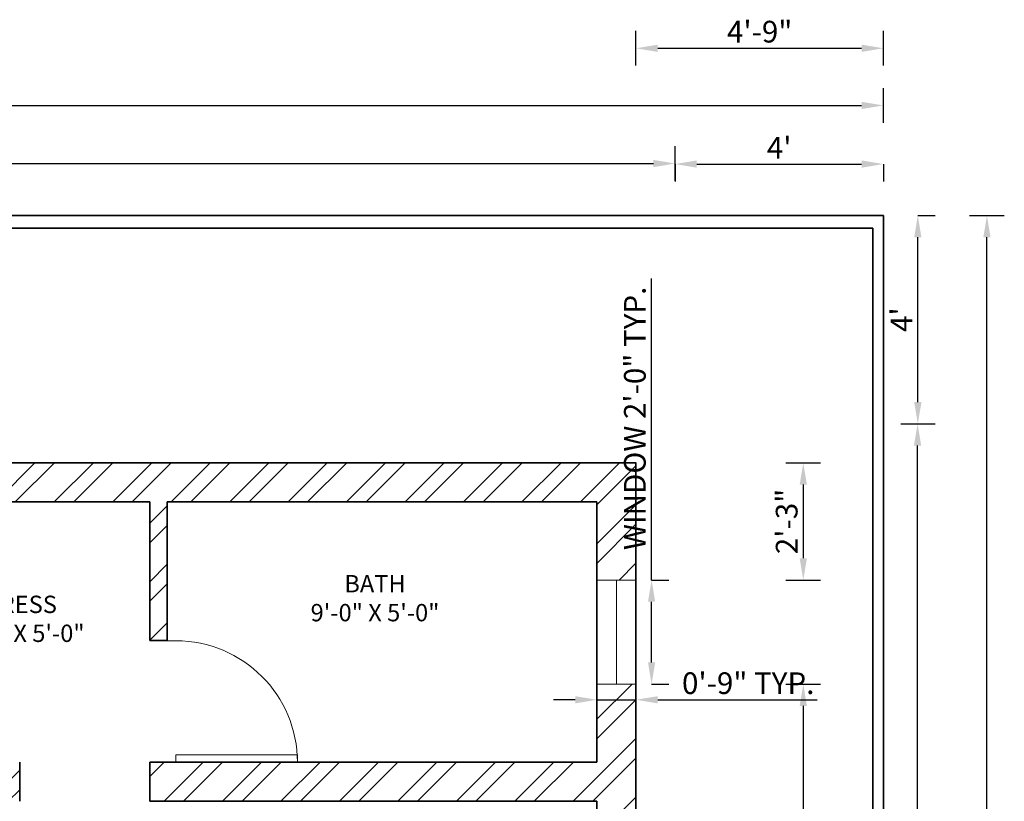
# Model space of a CAD drawing. Units: inches. Extents: x 468 to 1096, y 138 to 946.
# Tile 6 of 6: x 854 to 1081, y 766 to 946. Entities that reach past the tile are written whole.
import ezdxf

# ---------------------------------------------------------------- set-up
doc = ezdxf.new("R2010")
doc.units = ezdxf.units.IN
for name, color, linetype, lineweight in [('A-ANNO-DIMS', 2, 'Continuous', 18), ('A-AREA-IDEN', 7, 'Continuous', 18), ('A-DOOR', 3, 'Continuous', 18), ('A-GLAZ', 4, 'Continuous', 18), ('A-WALL', 7, 'Continuous', 35), ('A-WALL-PATT', 8, 'Continuous', 13), ('C-PROP', 7, 'Continuous', 35)]:
    doc.layers.add(name, color=color, linetype=linetype, lineweight=lineweight)
doc.styles.get("Standard").update_dxf_attribs({"font": 'arial.ttf'})
doc.dimstyles.new('ISO-25', dxfattribs={"dimtxt": 5, "dimasz": 5, "dimexe": 4, "dimexo": 4, "dimtad": 1, "dimdec": 1, "dimlunit": 3, "dimtxsty": 'Standard', "dimcen": 2.5, "dimadec": 0, "dimazin": 0, "dimtfac": 1, "dimtdec": 1, "dimtmove": 0, "dimatfit": 3, "dimfxl": 4, "dimfxlon": 1, "dimarcsym": 0})

# ---------------------------------------------------------------- blocks, each defined once
blk = doc.blocks.new('*U6')
for p, q in [((-28, 0), (-28, -6)), ((0, 0), (0, -6))]:
    blk.add_line(p, q)
blk.add_lwpolyline([(0, 0), (0, 28), (-1.75, 28), (-1.75, 0)], close=True)
blk.add_arc((0, 0), 28, 90, 180)
blk = doc.blocks.new('*D16')
at = {"layer": 'A-ANNO-DIMS', "color": 0, "lineweight": -2, "transparency": 16777216}
for p, q in [((639.13, 909.15), (639.13, 917.15)), ((1005.13, 909.15), (1005.13, 917.15)), ((644.13, 913.15), (1000.13, 913.15))]:
    blk.add_line(p, q, dxfattribs=at)
at = {"layer": 'A-ANNO-DIMS', "color": 0, "transparency": 16777216}
for points in [[(644.13, 913.98), (644.13, 912.31), (639.13, 913.15)], [(1000.13, 913.98), (1000.13, 912.31), (1005.13, 913.15)]]:
    blk.add_solid(points, dxfattribs=at)
at = {"layer": 'Defpoints', "color": 0, "transparency": 16777216}
for p in [(1005.13, 913.15), (639.13, 901.16), (1005.13, 901.16)]:
    blk.add_point(p, dxfattribs=at)
at = {"layer": 'A-ANNO-DIMS', "color": 0, "transparency": 16777216, "insert": (822.13, 916.33), "char_height": 5, "attachment_point": 5}
blk.add_mtext('30\'-6"', dxfattribs=at)
blk = doc.blocks.new('*D17')
at = {"layer": 'A-ANNO-DIMS', "color": 0, "lineweight": -2, "transparency": 16777216}
for p, q in [((1005.13, 913.03), (1005.13, 909.03)), ((1010.13, 913.03), (1048.13, 913.03)), ((1053.13, 913.03), (1053.13, 909.03))]:
    blk.add_line(p, q, dxfattribs=at)
at = {"layer": 'A-ANNO-DIMS', "color": 0, "transparency": 16777216}
for points in [[(1010.13, 913.86), (1010.13, 912.19), (1005.13, 913.03)], [(1048.13, 913.86), (1048.13, 912.19), (1053.13, 913.03)]]:
    blk.add_solid(points, dxfattribs=at)
at = {"layer": 'Defpoints', "color": 0, "transparency": 16777216}
for p in [(1005.13, 913.15), (1053.13, 913.15), (1053.13, 913.03)]:
    blk.add_point(p, dxfattribs=at)
at = {"layer": 'A-ANNO-DIMS', "color": 0, "transparency": 16777216, "insert": (1029.13, 916.15), "char_height": 5, "attachment_point": 5}
blk.add_mtext("4'", dxfattribs=at)
blk = doc.blocks.new('*D26')
at = {"layer": 'A-ANNO-DIMS', "color": 0, "lineweight": -2, "transparency": 16777216}
for p, q in [((1073, 901.16), (1081, 901.16)), ((1077, 186.16), (1077, 896.16)), ((1073, 181.16), (1081, 181.16))]:
    blk.add_line(p, q, dxfattribs=at)
at = {"layer": 'A-ANNO-DIMS', "color": 0, "transparency": 16777216}
for points in [[(1076.17, 896.16), (1077.83, 896.16), (1077, 901.16)], [(1076.17, 186.16), (1077.83, 186.16), (1077, 181.16)]]:
    blk.add_solid(points, dxfattribs=at)
at = {"layer": 'Defpoints', "color": 0, "transparency": 16777216}
for p in [(1053.13, 901.16), (1077, 901.16), (1053.13, 181.16)]:
    blk.add_point(p, dxfattribs=at)
at = {"layer": 'A-ANNO-DIMS', "color": 0, "transparency": 16777216, "insert": (1073.82, 541.16), "char_height": 5, "attachment_point": 5, "rotation": 90}
blk.add_mtext("60'", dxfattribs=at)
blk = doc.blocks.new('*D28')
at = {"layer": 'A-ANNO-DIMS', "color": 0, "lineweight": -2, "transparency": 16777216}
for p, q in [((1057.13, 853.16), (1065.02, 853.16)), ((1061.02, 417.16), (1061.02, 848.16)), ((1057.13, 412.16), (1065.02, 412.16))]:
    blk.add_line(p, q, dxfattribs=at)
at = {"layer": 'A-ANNO-DIMS', "color": 0, "transparency": 16777216}
for points in [[(1060.18, 848.16), (1061.85, 848.16), (1061.02, 853.16)], [(1060.18, 417.16), (1061.85, 417.16), (1061.02, 412.16)]]:
    blk.add_solid(points, dxfattribs=at)
at = {"layer": 'Defpoints', "color": 0, "transparency": 16777216}
for p in [(1053.13, 853.16), (1061.02, 853.16), (1053.13, 412.16)]:
    blk.add_point(p, dxfattribs=at)
at = {"layer": 'A-ANNO-DIMS', "color": 0, "transparency": 16777216, "insert": (1057.84, 632.66), "char_height": 5, "attachment_point": 5, "rotation": 90}
blk.add_mtext('36\'-9"', dxfattribs=at)
blk = doc.blocks.new('*D29')
at = {"layer": 'A-ANNO-DIMS', "color": 0, "lineweight": -2, "transparency": 16777216}
for p, q in [((1061.07, 901.16), (1065.07, 901.16)), ((1061.07, 858.16), (1061.07, 896.16)), ((1061.07, 853.16), (1065.07, 853.16))]:
    blk.add_line(p, q, dxfattribs=at)
at = {"layer": 'A-ANNO-DIMS', "color": 0, "transparency": 16777216}
for points in [[(1060.24, 896.16), (1061.91, 896.16), (1061.07, 901.16)], [(1060.24, 858.16), (1061.91, 858.16), (1061.07, 853.16)]]:
    blk.add_solid(points, dxfattribs=at)
at = {"layer": 'Defpoints', "color": 0, "transparency": 16777216}
for p in [(1061.02, 901.16), (1061.07, 901.16), (1061.02, 853.16)]:
    blk.add_point(p, dxfattribs=at)
at = {"layer": 'A-ANNO-DIMS', "color": 0, "transparency": 16777216, "insert": (1057.95, 877.16), "char_height": 5, "attachment_point": 5, "rotation": 90}
blk.add_mtext("4'", dxfattribs=at)
blk = doc.blocks.new('*D30')
at = {"layer": 'A-ANNO-DIMS', "color": 0, "lineweight": -2, "transparency": 16777216}
for p, q in [((513.13, 922.53), (513.13, 930.53)), ((1053.13, 922.53), (1053.13, 930.53)), ((518.13, 926.53), (1048.13, 926.53))]:
    blk.add_line(p, q, dxfattribs=at)
at = {"layer": 'A-ANNO-DIMS', "color": 0, "transparency": 16777216}
for points in [[(518.13, 927.37), (518.13, 925.7), (513.13, 926.53)], [(1048.13, 927.37), (1048.13, 925.7), (1053.13, 926.53)]]:
    blk.add_solid(points, dxfattribs=at)
at = {"layer": 'Defpoints', "color": 0, "transparency": 16777216}
for p in [(1053.13, 926.53), (513.13, 901.16), (1053.13, 901.16)]:
    blk.add_point(p, dxfattribs=at)
at = {"layer": 'A-ANNO-DIMS', "color": 0, "transparency": 16777216, "insert": (783.13, 929.7), "char_height": 5, "attachment_point": 5}
blk.add_mtext("45'", dxfattribs=at)
blk = doc.blocks.new('WIN-24-W9')
for p, q in [((0, 24), (9, 24)), ((4.5, 24), (4.5, 0)), ((0, 0), (9, 0))]:
    blk.add_line(p, q)
blk = doc.blocks.new('*D39')
at = {"layer": 'A-ANNO-DIMS', "color": 0, "lineweight": -2, "transparency": 16777216}
for p, q in [((999.73, 817.16), (999.73, 886.68)), ((999.73, 817.16), (1003.73, 817.16)), ((999.73, 798.16), (999.73, 812.16)), ((999.73, 793.16), (1003.73, 793.16))]:
    blk.add_line(p, q, dxfattribs=at)
at = {"layer": 'A-ANNO-DIMS', "color": 0, "transparency": 16777216}
for points in [[(998.9, 812.16), (1000.56, 812.16), (999.73, 817.16)], [(998.9, 798.16), (1000.56, 798.16), (999.73, 793.16)]]:
    blk.add_solid(points, dxfattribs=at)
at = {"layer": 'Defpoints', "color": 0, "transparency": 16777216}
for p in [(996.13, 817.16), (999.73, 817.16), (996.13, 793.16)]:
    blk.add_point(p, dxfattribs=at)
at = {"layer": 'A-ANNO-DIMS', "color": 0, "transparency": 16777216, "insert": (996.52, 854.42), "char_height": 5, "attachment_point": 5, "rotation": 90}
blk.add_mtext('WINDOW 2\'-0" TYP.', dxfattribs=at)
blk = doc.blocks.new('*D40')
at = {"layer": 'A-ANNO-DIMS', "color": 0, "lineweight": -2, "transparency": 16777216}
for p, q in [((982.13, 789.56), (977.13, 789.56)), ((987.13, 789.56), (987.13, 785.56)), ((987.13, 789.56), (996.13, 789.56)), ((996.13, 789.56), (996.13, 785.56)), ((1001.13, 789.56), (1037.86, 789.56))]:
    blk.add_line(p, q, dxfattribs=at)
at = {"layer": 'A-ANNO-DIMS', "color": 0, "transparency": 16777216}
for points in [[(982.13, 790.39), (982.13, 788.73), (987.13, 789.56)], [(1001.13, 790.39), (1001.13, 788.73), (996.13, 789.56)]]:
    blk.add_solid(points, dxfattribs=at)
at = {"layer": 'Defpoints', "color": 0, "transparency": 16777216}
for p in [(987.13, 793.16), (996.13, 793.16), (996.13, 789.56)]:
    blk.add_point(p, dxfattribs=at)
at = {"layer": 'A-ANNO-DIMS', "color": 0, "transparency": 16777216, "insert": (1021.99, 792.74), "char_height": 5, "attachment_point": 5}
blk.add_mtext('0\'-9" TYP.', dxfattribs=at)
blk = doc.blocks.new('*D65')
at = {"layer": 'A-ANNO-DIMS', "color": 0, "lineweight": -2, "transparency": 16777216}
for p, q in [((478.58, 803.16), (470.58, 803.16)), ((474.58, 780.16), (474.58, 798.16)), ((478.58, 775.16), (470.58, 775.16))]:
    blk.add_line(p, q, dxfattribs=at)
at = {"layer": 'A-ANNO-DIMS', "color": 0, "transparency": 16777216}
for points in [[(473.75, 798.16), (475.41, 798.16), (474.58, 803.16)], [(473.75, 780.16), (475.41, 780.16), (474.58, 775.16)]]:
    blk.add_solid(points, dxfattribs=at)
at = {"layer": 'Defpoints', "color": 0, "transparency": 16777216}
for p in [(474.58, 803.16), (884.13, 803.16), (884.13, 775.16)]:
    blk.add_point(p, dxfattribs=at)
at = {"layer": 'A-ANNO-DIMS', "color": 0, "transparency": 16777216, "insert": (471.44, 789.16), "char_height": 5, "attachment_point": 5, "rotation": 90}
blk.add_mtext('2\'-4"', dxfattribs=at)
blk = doc.blocks.new('*D71')
at = {"layer": 'A-ANNO-DIMS', "color": 0, "lineweight": -2, "transparency": 16777216}
for p, q in [((1030.68, 844.16), (1038.68, 844.16)), ((1034.68, 839.16), (1034.68, 822.16)), ((1030.68, 817.16), (1038.68, 817.16))]:
    blk.add_line(p, q, dxfattribs=at)
at = {"layer": 'A-ANNO-DIMS', "color": 0, "transparency": 16777216}
for points in [[(1033.85, 839.16), (1035.51, 839.16), (1034.68, 844.16)], [(1033.85, 822.16), (1035.51, 822.16), (1034.68, 817.16)]]:
    blk.add_solid(points, dxfattribs=at)
at = {"layer": 'Defpoints', "color": 0, "transparency": 16777216}
for p in [(996.13, 844.16), (996.13, 817.16), (1034.68, 817.16)]:
    blk.add_point(p, dxfattribs=at)
at = {"layer": 'A-ANNO-DIMS', "color": 0, "transparency": 16777216, "insert": (1031.5, 830.66), "char_height": 5, "attachment_point": 5, "rotation": 90}
blk.add_mtext('2\'-3"', dxfattribs=at)
blk = doc.blocks.new('*D72')
at = {"layer": 'A-ANNO-DIMS', "color": 0, "lineweight": -2, "transparency": 16777216}
for p, q in [((1030.68, 793.16), (1038.68, 793.16)), ((1034.68, 788.16), (1034.68, 723.16)), ((1030.68, 718.16), (1038.68, 718.16))]:
    blk.add_line(p, q, dxfattribs=at)
at = {"layer": 'A-ANNO-DIMS', "color": 0, "transparency": 16777216}
for points in [[(1033.85, 788.16), (1035.51, 788.16), (1034.68, 793.16)], [(1033.85, 723.16), (1035.51, 723.16), (1034.68, 718.16)]]:
    blk.add_solid(points, dxfattribs=at)
at = {"layer": 'Defpoints', "color": 0, "transparency": 16777216}
for p in [(996.13, 793.16), (996.13, 718.16), (1034.68, 718.16)]:
    blk.add_point(p, dxfattribs=at)
at = {"layer": 'A-ANNO-DIMS', "color": 0, "transparency": 16777216, "insert": (1031.5, 755.66), "char_height": 5, "attachment_point": 5, "rotation": 90}
blk.add_mtext('6\'-3"', dxfattribs=at)
blk = doc.blocks.new('*D74')
at = {"layer": 'A-ANNO-DIMS', "color": 0, "lineweight": -2, "transparency": 16777216}
for p, q in [((996.13, 935.71), (996.13, 943.71)), ((1053.13, 935.71), (1053.13, 943.71)), ((1001.13, 939.71), (1048.13, 939.71))]:
    blk.add_line(p, q, dxfattribs=at)
at = {"layer": 'A-ANNO-DIMS', "color": 0, "transparency": 16777216}
for points in [[(1001.13, 940.54), (1001.13, 938.88), (996.13, 939.71)], [(1048.13, 940.54), (1048.13, 938.88), (1053.13, 939.71)]]:
    blk.add_solid(points, dxfattribs=at)
at = {"layer": 'Defpoints', "color": 0, "transparency": 16777216}
for p in [(1053.13, 939.71), (1053.13, 901.16), (996.13, 844.16)]:
    blk.add_point(p, dxfattribs=at)
at = {"layer": 'A-ANNO-DIMS', "color": 0, "transparency": 16777216, "insert": (1024.63, 942.89), "char_height": 5, "attachment_point": 5}
blk.add_mtext('4\'-9"', dxfattribs=at)

msp = doc.modelspace()

# ---------------------------------------------------------------- hatches: boundary and pattern name
at = {"layer": 'A-WALL-PATT'}
h = msp.add_hatch(dxfattribs=at)
h.set_pattern_fill('ANSI32', color=256)
h.paths.add_polyline_path([(696.13, 634.16), (687.13, 634.16), (650.13, 634.16), (567.13, 634.16), (567.13, 625.16), (573.13, 625.16), (573.13, 610.16), (579.13, 610.16), (579.13, 625.16), (687.13, 625.16), (687.13, 454.16), (696.13, 454.16), (696.13, 598.16), (813.13, 598.16), (813.13, 607.16), (696.13, 607.16)])
h.paths.add_polyline_path([(777.13, 688.16), (777.13, 691.16), (696.13, 691.16), (696.13, 820.16), (721.13, 820.16), (721.13, 829.16), (687.13, 829.16), (687.13, 820.16), (687.13, 674.16), (696.13, 674.16), (696.13, 682.16), (777.13, 682.16)])
h.paths.add_polyline_path([(854.13, 775.16), (822.13, 775.16), (822.13, 835.16), (884.13, 835.16), (884.13, 803.19), (888.13, 803.19), (888.13, 835.16), (987.13, 835.16), (987.13, 817.16), (996.13, 817.16), (996.13, 844.16), (987.13, 844.16), (813.13, 844.16), (813.13, 829.16), (813.13, 823.16), (813.13, 791.16), (813.13, 691.16), (813.13, 688.16), (813.13, 682.16), (813.13, 643.16), (819.13, 643.16), (822.13, 643.16), (822.13, 691.16), (822.13, 766.16), (854.13, 766.16)])
h.paths.add_polyline_path([(996.13, 775.16), (996.13, 784.16), (996.13, 793.16), (987.13, 793.16), (987.13, 775.16), (884.13, 775.16), (884.13, 766.16), (987.13, 766.16), (987.13, 718.16), (996.13, 718.16)], flags=17)
h.paths.add_polyline_path([(781.13, 829.16), (757.13, 829.16), (757.13, 820.16), (781.13, 820.16)])

# ---------------------------------------------------------------- linework, layer by layer
at = {"layer": 'A-WALL'}
for p, q in [((822.13, 835.16), (884.13, 835.16)), ((884.13, 803.19), (884.13, 835.16)), ((888.13, 803.19), (888.13, 835.16)), ((888.13, 835.16), (987.13, 835.16)), ((987.13, 835.16), (987.13, 775.16)), ((884.13, 803.19), (888.13, 803.19)), ((854.13, 775.16), (854.13, 766.16)), ((884.13, 775.16), (884.13, 766.16)), ((884.13, 775.16), (987.13, 775.16)), ((884.13, 766.16), (987.13, 766.16)), ((987.13, 766.16), (987.13, 607.16))]:
    msp.add_line(p, q, dxfattribs=at)
msp.add_lwpolyline([(813.13, 829.16), (813.13, 844.16), (987.13, 844.16), (996.13, 844.16), (996.13, 784.16), (996.13, 775.16), (996.13, 607.16), (996.13, 598.16)], dxfattribs=at)
at = {"layer": 'C-PROP'}
for p, q in [((1053.13, 901.16), (513.13, 901.16)), ((1053.13, 181.16), (1053.13, 901.16)), ((1050.72, 898.26), (639.13, 898.26)), ((1050.72, 892.16), (1050.72, 898.26)), ((1050.72, 412.16), (1050.72, 892.16))]:
    msp.add_line(p, q, dxfattribs=at)

# ---------------------------------------------------------------- block references
at = {"layer": 'A-DOOR', "rotation": 270}
msp.add_blockref('*U6', (890.13, 775.16), dxfattribs=at)
at = {"layer": 'A-GLAZ'}
msp.add_blockref('WIN-24-W9', (987.13, 793.16), dxfattribs=at)

# ---------------------------------------------------------------- texts
at = {"layer": 'A-AREA-IDEN', "char_height": 4, "attachment_point": 1}
for s, insert in [('\\pxqc;BATH\\P9\'-0" X 5\'-0"', (917.87, 818.31)), ('\\pxqc;DRESS\\P5\'-2" X 5\'-0"', (836.11, 813.55))]:
    msp.add_mtext_dynamic_manual_height_columns(s, width=36.2598, gutter_width=12.5, heights=[0], dxfattribs=dict(at, insert=insert))

# ---------------------------------------------------------------- dimensions: what is measured, and where the dimension line sits
at = {"layer": 'A-ANNO-DIMS'}
for base, p1, p2, override, picture, middle in [((1053.13, 939.71), (996.13, 844.16), (1053.13, 901.16), {"dimdec": 1, "dimlfac": 1, "dimrnd": 0, "dimzin": 1, "dimdsep": 46, "dimlunit": 4, "dimfrac": 2}, '*D74', (1024.63, 942.89)), ((1053.13, 926.53), (513.13, 901.16), (1053.13, 901.16), {"dimclrd": 0, "dimclre": 0, "dimclrt": 0}, '*D30', (783.13, 929.7)), ((1005.13, 913.15), (639.13, 901.16), (1005.13, 901.16), {"dimclrd": 0, "dimclre": 0, "dimclrt": 0}, '*D16', (822.13, 916.33)), ((1053.13, 913.03), (1005.13, 913.15), (1053.13, 913.15), {"dimclrd": 0, "dimclre": 0, "dimclrt": 0}, '*D17', (1029.13, 916.15))]:
    dim = msp.add_linear_dim(base=base, p1=p1, p2=p2, dimstyle='ISO-25', override=override, dxfattribs=at)
    dim.commit()
    dim.dimension.update_dxf_attribs({"geometry": picture, "text_midpoint": middle})
for base, p1, p2, angle, override, picture, middle in [((1077, 901.16), (1053.13, 181.16), (1053.13, 901.16), 90, {"dimclrd": 0, "dimclre": 0, "dimclrt": 0}, '*D26', (1073.82, 541.16)), ((1061.07, 901.16), (1061.02, 853.16), (1061.02, 901.16), 90, {"dimclrd": 0, "dimclre": 0, "dimclrt": 0}, '*D29', (1057.95, 877.16)), ((1061.02, 853.16), (1053.13, 412.16), (1053.13, 853.16), 90, {"dimclrd": 0, "dimclre": 0, "dimclrt": 0}, '*D28', (1057.84, 632.66)), ((1034.68, 817.16), (996.13, 844.16), (996.13, 817.16), 270, {"dimdec": 1, "dimlfac": 1, "dimrnd": 0, "dimzin": 1, "dimdsep": 46, "dimlunit": 4, "dimfrac": 2}, '*D71', (1031.5, 830.66)), ((474.58, 803.16), (884.13, 775.16), (884.13, 803.16), 90, {"dimdec": 1, "dimlfac": 1, "dimrnd": 0, "dimzin": 1, "dimdsep": 46, "dimlunit": 4, "dimfrac": 2}, '*D65', (471.44, 789.16)), ((1034.68, 718.16), (996.13, 793.16), (996.13, 718.16), 270, {"dimdec": 1, "dimlfac": 1, "dimrnd": 0, "dimzin": 1, "dimdsep": 46, "dimlunit": 4, "dimfrac": 2}, '*D72', (1031.5, 755.66))]:
    dim = msp.add_linear_dim(base=base, p1=p1, p2=p2, angle=angle, dimstyle='ISO-25', override=override, dxfattribs=at)
    dim.commit()
    dim.dimension.update_dxf_attribs({"geometry": picture, "text_midpoint": middle})
dim = msp.add_linear_dim(base=(999.73, 817.16), p1=(996.13, 793.16), p2=(996.13, 817.16), angle=90, text='WINDOW <> TYP.', dimstyle='ISO-25', override={"dimdec": 1, "dimlfac": 1, "dimrnd": 0, "dimzin": 1, "dimdsep": 46, "dimlunit": 4, "dimfrac": 2}, dxfattribs=at)
dim.commit()
dim.dimension.update_dxf_attribs({"geometry": '*D39', "text_midpoint": (996.52, 854.42)})
dim = msp.add_linear_dim(base=(996.13, 789.56), p1=(987.13, 793.16), p2=(996.13, 793.16), text='<> TYP.', dimstyle='ISO-25', override={"dimdec": 1, "dimlfac": 1, "dimrnd": 0, "dimzin": 1, "dimdsep": 46, "dimlunit": 4, "dimfrac": 2}, dxfattribs=at)
dim.commit()
dim.dimension.update_dxf_attribs({"geometry": '*D40', "text_midpoint": (1021.99, 792.74)})

doc.saveas('drawing.dxf')
